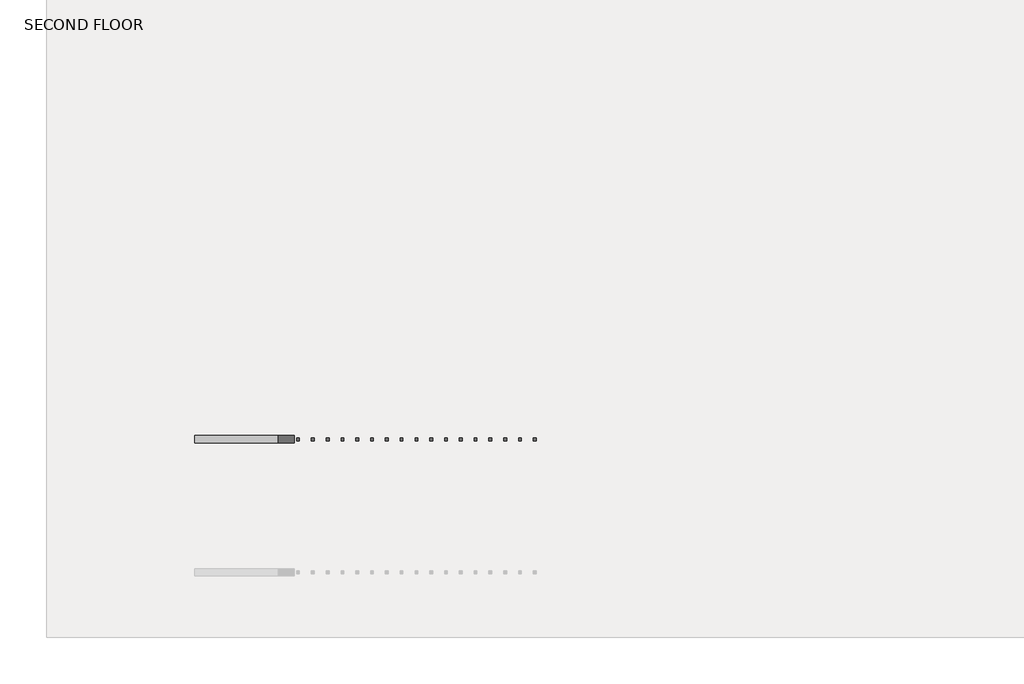
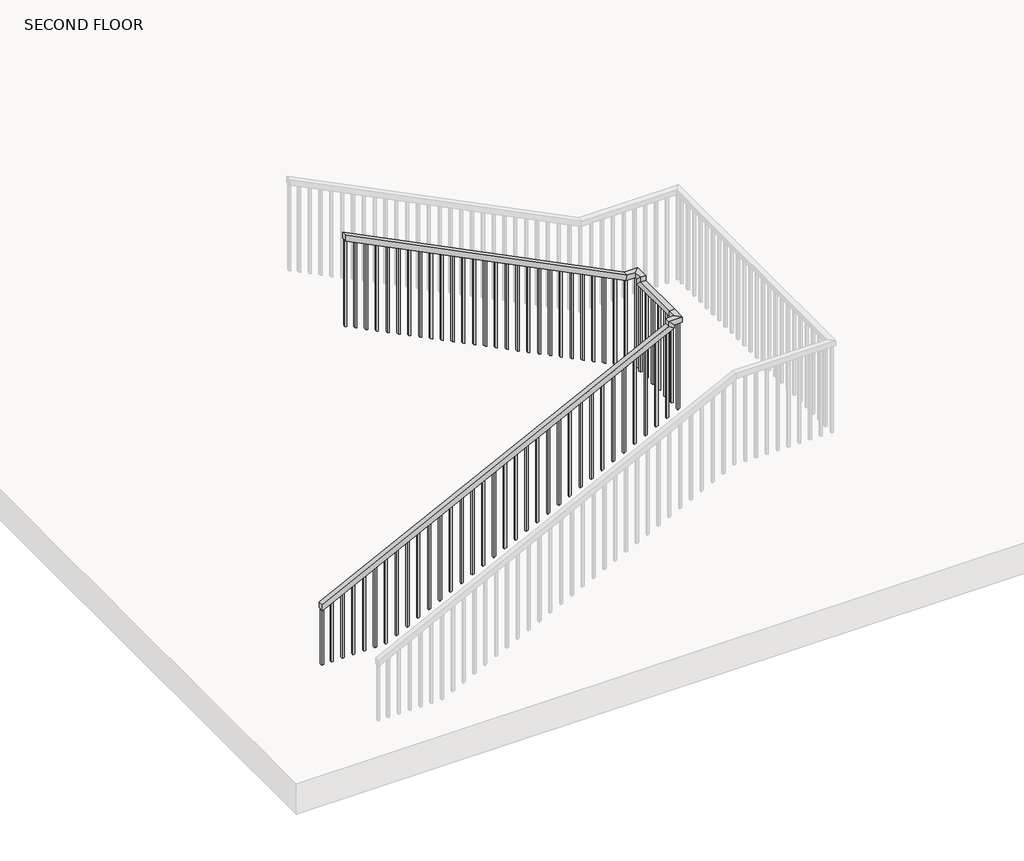
# One storey, part 2 of 2: 1 railing.
"""IFC4 building model written with IfcOpenShell, lengths in millimetres."""

from ifc_helpers import new_model, si_unit, frame, origin, place, context, project, spatial, polyline, outline, extrude, faceted_brep, element, save

model = new_model("IFC4")

# Units and contexts
model_context = context("Model", 3, world=origin())
ifc_project = project(units=[si_unit("LENGTHUNIT", "METRE", prefix="MILLI")], contexts=[model_context])

# Site, building, storey
site = spatial("IfcSite", under=ifc_project)
building = spatial("IfcBuilding", under=site)
storey = spatial("IfcBuildingStorey", under=building, Name="SECOND FLOOR", Elevation=6096.0)

# Railing
placement = place(None, origin())
element("IfcRailing", 1, ObjectType="Handrail - Rectangular", at=placement, inside=storey, context=model_context, shape_type="SolidModel", body=[
    faceted_brep([(-8362.2800418, -4455.7090076, 7010.4), (-8362.2800418, -4455.7090076, 6953.6038734), (-8362.2800418, -4506.5090076, 6953.6038734), (-8362.2800418, -4506.5090076, 7010.4), (-5111.0800418, -4455.7090076, 8636.0), (-5060.2800418, -4455.7090076, 8604.6038734), (-5060.2800418, -4506.5090076, 8604.6038734), (-5111.0800418, -4506.5090076, 8636.0), (-5111.0800418, -4455.7090076, 8686.8), (-5060.2800418, -4455.7090076, 8636.0), (-5060.2800418, -4506.5090076, 8636.0), (-5111.0800418, -4506.5090076, 8686.8), (-5034.8800418, -4455.7090076, 8686.8), (-5034.8800418, -4455.7090076, 8636.0), (-4984.0800418, -4506.5090076, 8636.0), (-4984.0800418, -4506.5090076, 8686.8), (-5034.8800418, -4379.5090076, 8686.8), (-5034.8800418, -4379.5090076, 8636.0), (-4984.0800418, -4379.5090076, 8636.0), (-4984.0800418, -4379.5090076, 8686.8), (-5034.8800418, -3907.7346494, 8686.8), (-5034.8800418, -3856.9346494, 8636.0), (-4984.0800418, -3856.9346494, 8636.0), (-4984.0800418, -3907.7346494, 8686.8), (-5034.8800418, -3907.7346494, 8737.6), (-5034.8800418, -3856.9346494, 8686.8), (-4984.0800418, -3856.9346494, 8686.8), (-4984.0800418, -3907.7346494, 8737.6), (-5034.8800418, -3831.5346494, 8737.6), (-5034.8800418, -3831.5346494, 8686.8), (-4984.0800418, -3780.7346494, 8686.8), (-4984.0800418, -3780.7346494, 8737.6), (-5111.0800418, -3831.5346494, 8737.6), (-5123.072295, -3831.5346494, 8686.8), (-5123.072295, -3780.7346494, 8686.8), (-5111.0800418, -3780.7346494, 8737.6), (-7752.6800418, -3831.5346494, 10058.4), (-7752.6800418, -3780.7346494, 10058.4), (-7752.6800418, -3780.7346494, 10001.6038734), (-7752.6800418, -3831.5346494, 10001.6038734)], [[[0, 1, 2, 3]], [[1, 0, 4, 5]], [[2, 1, 5, 6]], [[3, 2, 6, 7]], [[0, 3, 7, 4]], [[5, 4, 8, 9]], [[6, 5, 9, 10]], [[7, 6, 10, 11]], [[4, 7, 11, 8]], [[9, 8, 12, 13]], [[10, 9, 13, 14]], [[11, 10, 14, 15]], [[8, 11, 15, 12]], [[13, 12, 16, 17]], [[14, 13, 17, 18]], [[15, 14, 18, 19]], [[12, 15, 19, 16]], [[17, 16, 20, 21]], [[18, 17, 21, 22]], [[19, 18, 22, 23]], [[16, 19, 23, 20]], [[21, 20, 24, 25]], [[22, 21, 25, 26]], [[23, 22, 26, 27]], [[20, 23, 27, 24]], [[25, 24, 28, 29]], [[26, 25, 29, 30]], [[27, 26, 30, 31]], [[24, 27, 31, 28]], [[29, 28, 32, 33]], [[30, 29, 33, 34]], [[31, 30, 34, 35]], [[28, 31, 35, 32]], [[36, 37, 38, 39]], [[33, 32, 36, 39]], [[34, 33, 39, 38]], [[35, 34, 38, 37]], [[32, 35, 37, 36]]]),
    extrude(outline(polyline([(9946.0413734, -7641.5550418), (9955.5663734, -7660.6050418), (9097.9625, -7660.6050418), (9088.4375, -7641.5550418), (9946.0413734, -7641.5550418)])), frame((0.0, -3815.6596494, 0.0), z_axis=(0.0, 1.0, 0.0), x_axis=(0.0, 0.0, 1.0)), (0.0, 0.0, 1.0), 19.05),
    extrude(outline(polyline([(9895.2413734, -7539.9550418), (9904.7663734, -7559.0050418), (9047.1625, -7559.0050418), (9037.6375, -7539.9550418), (9895.2413734, -7539.9550418)])), frame((0.0, -3815.6596494, 0.0), z_axis=(0.0, 1.0, 0.0), x_axis=(0.0, 0.0, 1.0)), (0.0, 0.0, 1.0), 19.05),
    extrude(outline(polyline([(9844.4413734, -7438.3550418), (9853.9663734, -7457.4050418), (8996.3625, -7457.4050418), (8986.8375, -7438.3550418), (9844.4413734, -7438.3550418)])), frame((0.0, -3815.6596494, 0.0), z_axis=(0.0, 1.0, 0.0), x_axis=(0.0, 0.0, 1.0)), (0.0, 0.0, 1.0), 19.05),
    extrude(outline(polyline([(9793.6413734, -7336.7550418), (9803.1663734, -7355.8050418), (8945.5625, -7355.8050418), (8936.0375, -7336.7550418), (9793.6413734, -7336.7550418)])), frame((0.0, -3815.6596494, 0.0), z_axis=(0.0, 1.0, 0.0), x_axis=(0.0, 0.0, 1.0)), (0.0, 0.0, 1.0), 19.05),
    extrude(outline(polyline([(9742.8413734, -7235.1550418), (9752.3663734, -7254.2050418), (8894.7625, -7254.2050418), (8885.2375, -7235.1550418), (9742.8413734, -7235.1550418)])), frame((0.0, -3815.6596494, 0.0), z_axis=(0.0, 1.0, 0.0), x_axis=(0.0, 0.0, 1.0)), (0.0, 0.0, 1.0), 19.05),
    extrude(outline(polyline([(9692.0413734, -7133.5550418), (9701.5663734, -7152.6050418), (8843.9625, -7152.6050418), (8834.4375, -7133.5550418), (9692.0413734, -7133.5550418)])), frame((0.0, -3815.6596494, 0.0), z_axis=(0.0, 1.0, 0.0), x_axis=(0.0, 0.0, 1.0)), (0.0, 0.0, 1.0), 19.05),
    extrude(outline(polyline([(9641.2413734, -7031.9550418), (9650.7663734, -7051.0050418), (8793.1625, -7051.0050418), (8783.6375, -7031.9550418), (9641.2413734, -7031.9550418)])), frame((0.0, -3815.6596494, 0.0), z_axis=(0.0, 1.0, 0.0), x_axis=(0.0, 0.0, 1.0)), (0.0, 0.0, 1.0), 19.05),
    extrude(outline(polyline([(9590.4413734, -6930.3550418), (9599.9663734, -6949.4050418), (8742.3625, -6949.4050418), (8732.8375, -6930.3550418), (9590.4413734, -6930.3550418)])), frame((0.0, -3815.6596494, 0.0), z_axis=(0.0, 1.0, 0.0), x_axis=(0.0, 0.0, 1.0)), (0.0, 0.0, 1.0), 19.05),
    extrude(outline(polyline([(9539.6413734, -6828.7550418), (9549.1663734, -6847.8050418), (8691.5625, -6847.8050418), (8682.0375, -6828.7550418), (9539.6413734, -6828.7550418)])), frame((0.0, -3815.6596494, 0.0), z_axis=(0.0, 1.0, 0.0), x_axis=(0.0, 0.0, 1.0)), (0.0, 0.0, 1.0), 19.05),
    extrude(outline(polyline([(9488.8413734, -6727.1550418), (9498.3663734, -6746.2050418), (8640.7625, -6746.2050418), (8631.2375, -6727.1550418), (9488.8413734, -6727.1550418)])), frame((0.0, -3815.6596494, 0.0), z_axis=(0.0, 1.0, 0.0), x_axis=(0.0, 0.0, 1.0)), (0.0, 0.0, 1.0), 19.05),
    extrude(outline(polyline([(9438.0413734, -6625.5550418), (9447.5663734, -6644.6050418), (8589.9625, -6644.6050418), (8580.4375, -6625.5550418), (9438.0413734, -6625.5550418)])), frame((0.0, -3815.6596494, 0.0), z_axis=(0.0, 1.0, 0.0), x_axis=(0.0, 0.0, 1.0)), (0.0, 0.0, 1.0), 19.05),
    extrude(outline(polyline([(9387.2413734, -6523.9550418), (9396.7663734, -6543.0050418), (8539.1625, -6543.0050418), (8529.6375, -6523.9550418), (9387.2413734, -6523.9550418)])), frame((0.0, -3815.6596494, 0.0), z_axis=(0.0, 1.0, 0.0), x_axis=(0.0, 0.0, 1.0)), (0.0, 0.0, 1.0), 19.05),
    extrude(outline(polyline([(9336.4413734, -6422.3550418), (9345.9663734, -6441.4050418), (8488.3625, -6441.4050418), (8478.8375, -6422.3550418), (9336.4413734, -6422.3550418)])), frame((0.0, -3815.6596494, 0.0), z_axis=(0.0, 1.0, 0.0), x_axis=(0.0, 0.0, 1.0)), (0.0, 0.0, 1.0), 19.05),
    extrude(outline(polyline([(9285.6413734, -6320.7550418), (9295.1663734, -6339.8050418), (8437.5625, -6339.8050418), (8428.0375, -6320.7550418), (9285.6413734, -6320.7550418)])), frame((0.0, -3815.6596494, 0.0), z_axis=(0.0, 1.0, 0.0), x_axis=(0.0, 0.0, 1.0)), (0.0, 0.0, 1.0), 19.05),
    extrude(outline(polyline([(9234.8413734, -6219.1550418), (9244.3663734, -6238.2050418), (8386.7625, -6238.2050418), (8377.2375, -6219.1550418), (9234.8413734, -6219.1550418)])), frame((0.0, -3815.6596494, 0.0), z_axis=(0.0, 1.0, 0.0), x_axis=(0.0, 0.0, 1.0)), (0.0, 0.0, 1.0), 19.05),
    extrude(outline(polyline([(9184.0413734, -6117.5550418), (9193.5663734, -6136.6050418), (8335.9625, -6136.6050418), (8326.4375, -6117.5550418), (9184.0413734, -6117.5550418)])), frame((0.0, -3815.6596494, 0.0), z_axis=(0.0, 1.0, 0.0), x_axis=(0.0, 0.0, 1.0)), (0.0, 0.0, 1.0), 19.05),
    extrude(outline(polyline([(9133.2413734, -6015.9550418), (9142.7663734, -6035.0050418), (8285.1625, -6035.0050418), (8275.6375, -6015.9550418), (9133.2413734, -6015.9550418)])), frame((0.0, -3815.6596494, 0.0), z_axis=(0.0, 1.0, 0.0), x_axis=(0.0, 0.0, 1.0)), (0.0, 0.0, 1.0), 19.05),
    extrude(outline(polyline([(9082.4413734, -5914.3550418), (9091.9663734, -5933.4050418), (8234.3625, -5933.4050418), (8224.8375, -5914.3550418), (9082.4413734, -5914.3550418)])), frame((0.0, -3815.6596494, 0.0), z_axis=(0.0, 1.0, 0.0), x_axis=(0.0, 0.0, 1.0)), (0.0, 0.0, 1.0), 19.05),
    extrude(outline(polyline([(9031.6413734, -5812.7550418), (9041.1663734, -5831.8050418), (8183.5625, -5831.8050418), (8174.0375, -5812.7550418), (9031.6413734, -5812.7550418)])), frame((0.0, -3815.6596494, 0.0), z_axis=(0.0, 1.0, 0.0), x_axis=(0.0, 0.0, 1.0)), (0.0, 0.0, 1.0), 19.05),
    extrude(outline(polyline([(8980.8413734, -5711.1550418), (8990.3663734, -5730.2050418), (8132.7625, -5730.2050418), (8123.2375, -5711.1550418), (8980.8413734, -5711.1550418)])), frame((0.0, -3815.6596494, 0.0), z_axis=(0.0, 1.0, 0.0), x_axis=(0.0, 0.0, 1.0)), (0.0, 0.0, 1.0), 19.05),
    extrude(outline(polyline([(8930.0413734, -5609.5550418), (8939.5663734, -5628.6050418), (8081.9625, -5628.6050418), (8072.4375, -5609.5550418), (8930.0413734, -5609.5550418)])), frame((0.0, -3815.6596494, 0.0), z_axis=(0.0, 1.0, 0.0), x_axis=(0.0, 0.0, 1.0)), (0.0, 0.0, 1.0), 19.05),
    extrude(outline(polyline([(8879.2413734, -5507.9550418), (8888.7663734, -5527.0050418), (8031.1625, -5527.0050418), (8021.6375, -5507.9550418), (8879.2413734, -5507.9550418)])), frame((0.0, -3815.6596494, 0.0), z_axis=(0.0, 1.0, 0.0), x_axis=(0.0, 0.0, 1.0)), (0.0, 0.0, 1.0), 19.05),
    extrude(outline(polyline([(8828.4413734, -5406.3550418), (8837.9663734, -5425.4050418), (7980.3625, -5425.4050418), (7970.8375, -5406.3550418), (8828.4413734, -5406.3550418)])), frame((0.0, -3815.6596494, 0.0), z_axis=(0.0, 1.0, 0.0), x_axis=(0.0, 0.0, 1.0)), (0.0, 0.0, 1.0), 19.05),
    extrude(outline(polyline([(8777.6413734, -5304.7550418), (8787.1663734, -5323.8050418), (7929.5625, -5323.8050418), (7920.0375, -5304.7550418), (8777.6413734, -5304.7550418)])), frame((0.0, -3815.6596494, 0.0), z_axis=(0.0, 1.0, 0.0), x_axis=(0.0, 0.0, 1.0)), (0.0, 0.0, 1.0), 19.05),
    extrude(outline(polyline([(8726.8413734, -5203.1550418), (8736.3663734, -5222.2050418), (7878.7625, -5222.2050418), (7869.2375, -5203.1550418), (8726.8413734, -5203.1550418)])), frame((0.0, -3815.6596494, 0.0), z_axis=(0.0, 1.0, 0.0), x_axis=(0.0, 0.0, 1.0)), (0.0, 0.0, 1.0), 19.05),
    extrude(outline(polyline([(8686.8, -5101.5550418), (8686.8, -5120.6050418), (7827.9625, -5120.6050418), (7818.4375, -5101.5550418), (8686.8, -5101.5550418)])), frame((0.0, -3815.6596494, 0.0), z_axis=(0.0, 1.0, 0.0), x_axis=(0.0, 0.0, 1.0)), (0.0, 0.0, 1.0), 19.05),
    extrude(outline(polyline([(-4999.9550418, -3881.0340076), (-5019.0050418, -3881.0340076), (-5019.0050418, -3861.9840076), (-4999.9550418, -3861.9840076), (-4999.9550418, -3881.0340076)])), frame((0.0, 0.0, 7772.4), z_axis=(0.0, 0.0, 1.0), x_axis=(1.0, 0.0, 0.0)), (0.0, 0.0, 1.0), 863.6),
    extrude(outline(polyline([(-4999.9550418, -3982.6340076), (-5019.0050418, -3982.6340076), (-5019.0050418, -3963.5840076), (-4999.9550418, -3963.5840076), (-4999.9550418, -3982.6340076)])), frame((0.0, 0.0, 7772.4), z_axis=(0.0, 0.0, 1.0), x_axis=(1.0, 0.0, 0.0)), (0.0, 0.0, 1.0), 863.6),
    extrude(outline(polyline([(-4999.9550418, -4084.2340076), (-5019.0050418, -4084.2340076), (-5019.0050418, -4065.1840076), (-4999.9550418, -4065.1840076), (-4999.9550418, -4084.2340076)])), frame((0.0, 0.0, 7772.4), z_axis=(0.0, 0.0, 1.0), x_axis=(1.0, 0.0, 0.0)), (0.0, 0.0, 1.0), 863.6),
    extrude(outline(polyline([(-4999.9550418, -4185.8340076), (-5019.0050418, -4185.8340076), (-5019.0050418, -4166.7840076), (-4999.9550418, -4166.7840076), (-4999.9550418, -4185.8340076)])), frame((0.0, 0.0, 7772.4), z_axis=(0.0, 0.0, 1.0), x_axis=(1.0, 0.0, 0.0)), (0.0, 0.0, 1.0), 863.6),
    extrude(outline(polyline([(-4999.9550418, -4287.4340076), (-5019.0050418, -4287.4340076), (-5019.0050418, -4268.3840076), (-4999.9550418, -4268.3840076), (-4999.9550418, -4287.4340076)])), frame((0.0, 0.0, 7772.4), z_axis=(0.0, 0.0, 1.0), x_axis=(1.0, 0.0, 0.0)), (0.0, 0.0, 1.0), 863.6),
    extrude(outline(polyline([(-4999.9550418, -4389.0340076), (-5019.0050418, -4389.0340076), (-5019.0050418, -4369.9840076), (-4999.9550418, -4369.9840076), (-4999.9550418, -4389.0340076)])), frame((0.0, 0.0, 7772.4), z_axis=(0.0, 0.0, 1.0), x_axis=(1.0, 0.0, 0.0)), (0.0, 0.0, 1.0), 863.6),
    extrude(outline(polyline([(8583.9663734, -5101.5550418), (8574.4413734, -5120.6050418), (7716.8375, -5120.6050418), (7726.3625, -5101.5550418), (8583.9663734, -5101.5550418)])), frame((0.0, -4490.6340076, 0.0), z_axis=(0.0, 1.0, 0.0), x_axis=(0.0, 0.0, 1.0)), (0.0, 0.0, 1.0), 19.05),
    extrude(outline(polyline([(8533.1663734, -5203.1550418), (8523.6413734, -5222.2050418), (7666.0375, -5222.2050418), (7675.5625, -5203.1550418), (8533.1663734, -5203.1550418)])), frame((0.0, -4490.6340076, 0.0), z_axis=(0.0, 1.0, 0.0), x_axis=(0.0, 0.0, 1.0)), (0.0, 0.0, 1.0), 19.05),
    extrude(outline(polyline([(8482.3663734, -5304.7550418), (8472.8413734, -5323.8050418), (7615.2375, -5323.8050418), (7624.7625, -5304.7550418), (8482.3663734, -5304.7550418)])), frame((0.0, -4490.6340076, 0.0), z_axis=(0.0, 1.0, 0.0), x_axis=(0.0, 0.0, 1.0)), (0.0, 0.0, 1.0), 19.05),
    extrude(outline(polyline([(8431.5663734, -5406.3550418), (8422.0413734, -5425.4050418), (7564.4375, -5425.4050418), (7573.9625, -5406.3550418), (8431.5663734, -5406.3550418)])), frame((0.0, -4490.6340076, 0.0), z_axis=(0.0, 1.0, 0.0), x_axis=(0.0, 0.0, 1.0)), (0.0, 0.0, 1.0), 19.05),
    extrude(outline(polyline([(8380.7663734, -5507.9550418), (8371.2413734, -5527.0050418), (7513.6375, -5527.0050418), (7523.1625, -5507.9550418), (8380.7663734, -5507.9550418)])), frame((0.0, -4490.6340076, 0.0), z_axis=(0.0, 1.0, 0.0), x_axis=(0.0, 0.0, 1.0)), (0.0, 0.0, 1.0), 19.05),
    extrude(outline(polyline([(8329.9663734, -5609.5550418), (8320.4413734, -5628.6050418), (7462.8375, -5628.6050418), (7472.3625, -5609.5550418), (8329.9663734, -5609.5550418)])), frame((0.0, -4490.6340076, 0.0), z_axis=(0.0, 1.0, 0.0), x_axis=(0.0, 0.0, 1.0)), (0.0, 0.0, 1.0), 19.05),
    extrude(outline(polyline([(8279.1663734, -5711.1550418), (8269.6413734, -5730.2050418), (7412.0375, -5730.2050418), (7421.5625, -5711.1550418), (8279.1663734, -5711.1550418)])), frame((0.0, -4490.6340076, 0.0), z_axis=(0.0, 1.0, 0.0), x_axis=(0.0, 0.0, 1.0)), (0.0, 0.0, 1.0), 19.05),
    extrude(outline(polyline([(8228.3663734, -5812.7550418), (8218.8413734, -5831.8050418), (7361.2375, -5831.8050418), (7370.7625, -5812.7550418), (8228.3663734, -5812.7550418)])), frame((0.0, -4490.6340076, 0.0), z_axis=(0.0, 1.0, 0.0), x_axis=(0.0, 0.0, 1.0)), (0.0, 0.0, 1.0), 19.05),
    extrude(outline(polyline([(8177.5663734, -5914.3550418), (8168.0413734, -5933.4050418), (7310.4375, -5933.4050418), (7319.9625, -5914.3550418), (8177.5663734, -5914.3550418)])), frame((0.0, -4490.6340076, 0.0), z_axis=(0.0, 1.0, 0.0), x_axis=(0.0, 0.0, 1.0)), (0.0, 0.0, 1.0), 19.05),
    extrude(outline(polyline([(8126.7663734, -6015.9550418), (8117.2413734, -6035.0050418), (7259.6375, -6035.0050418), (7269.1625, -6015.9550418), (8126.7663734, -6015.9550418)])), frame((0.0, -4490.6340076, 0.0), z_axis=(0.0, 1.0, 0.0), x_axis=(0.0, 0.0, 1.0)), (0.0, 0.0, 1.0), 19.05),
    extrude(outline(polyline([(8075.9663734, -6117.5550418), (8066.4413734, -6136.6050418), (7208.8375, -6136.6050418), (7218.3625, -6117.5550418), (8075.9663734, -6117.5550418)])), frame((0.0, -4490.6340076, 0.0), z_axis=(0.0, 1.0, 0.0), x_axis=(0.0, 0.0, 1.0)), (0.0, 0.0, 1.0), 19.05),
    extrude(outline(polyline([(8025.1663734, -6219.1550418), (8015.6413734, -6238.2050418), (7158.0375, -6238.2050418), (7167.5625, -6219.1550418), (8025.1663734, -6219.1550418)])), frame((0.0, -4490.6340076, 0.0), z_axis=(0.0, 1.0, 0.0), x_axis=(0.0, 0.0, 1.0)), (0.0, 0.0, 1.0), 19.05),
    extrude(outline(polyline([(7974.3663734, -6320.7550418), (7964.8413734, -6339.8050418), (7107.2375, -6339.8050418), (7116.7625, -6320.7550418), (7974.3663734, -6320.7550418)])), frame((0.0, -4490.6340076, 0.0), z_axis=(0.0, 1.0, 0.0), x_axis=(0.0, 0.0, 1.0)), (0.0, 0.0, 1.0), 19.05),
    extrude(outline(polyline([(7923.5663734, -6422.3550418), (7914.0413734, -6441.4050418), (7056.4375, -6441.4050418), (7065.9625, -6422.3550418), (7923.5663734, -6422.3550418)])), frame((0.0, -4490.6340076, 0.0), z_axis=(0.0, 1.0, 0.0), x_axis=(0.0, 0.0, 1.0)), (0.0, 0.0, 1.0), 19.05),
    extrude(outline(polyline([(7872.7663734, -6523.9550418), (7863.2413734, -6543.0050418), (7005.6375, -6543.0050418), (7015.1625, -6523.9550418), (7872.7663734, -6523.9550418)])), frame((0.0, -4490.6340076, 0.0), z_axis=(0.0, 1.0, 0.0), x_axis=(0.0, 0.0, 1.0)), (0.0, 0.0, 1.0), 19.05),
    extrude(outline(polyline([(7821.9663734, -6625.5550418), (7812.4413734, -6644.6050418), (6954.8375, -6644.6050418), (6964.3625, -6625.5550418), (7821.9663734, -6625.5550418)])), frame((0.0, -4490.6340076, 0.0), z_axis=(0.0, 1.0, 0.0), x_axis=(0.0, 0.0, 1.0)), (0.0, 0.0, 1.0), 19.05),
    extrude(outline(polyline([(7771.1663734, -6727.1550418), (7761.6413734, -6746.2050418), (6904.0375, -6746.2050418), (6913.5625, -6727.1550418), (7771.1663734, -6727.1550418)])), frame((0.0, -4490.6340076, 0.0), z_axis=(0.0, 1.0, 0.0), x_axis=(0.0, 0.0, 1.0)), (0.0, 0.0, 1.0), 19.05),
    extrude(outline(polyline([(7720.3663734, -6828.7550418), (7710.8413734, -6847.8050418), (6853.2375, -6847.8050418), (6862.7625, -6828.7550418), (7720.3663734, -6828.7550418)])), frame((0.0, -4490.6340076, 0.0), z_axis=(0.0, 1.0, 0.0), x_axis=(0.0, 0.0, 1.0)), (0.0, 0.0, 1.0), 19.05),
    extrude(outline(polyline([(7669.5663734, -6930.3550418), (7660.0413734, -6949.4050418), (6802.4375, -6949.4050418), (6811.9625, -6930.3550418), (7669.5663734, -6930.3550418)])), frame((0.0, -4490.6340076, 0.0), z_axis=(0.0, 1.0, 0.0), x_axis=(0.0, 0.0, 1.0)), (0.0, 0.0, 1.0), 19.05),
    extrude(outline(polyline([(7618.7663734, -7031.9550418), (7609.2413734, -7051.0050418), (6751.6375, -7051.0050418), (6761.1625, -7031.9550418), (7618.7663734, -7031.9550418)])), frame((0.0, -4490.6340076, 0.0), z_axis=(0.0, 1.0, 0.0), x_axis=(0.0, 0.0, 1.0)), (0.0, 0.0, 1.0), 19.05),
    extrude(outline(polyline([(7567.9663734, -7133.5550418), (7558.4413734, -7152.6050418), (6700.8375, -7152.6050418), (6710.3625, -7133.5550418), (7567.9663734, -7133.5550418)])), frame((0.0, -4490.6340076, 0.0), z_axis=(0.0, 1.0, 0.0), x_axis=(0.0, 0.0, 1.0)), (0.0, 0.0, 1.0), 19.05),
    extrude(outline(polyline([(7517.1663734, -7235.1550418), (7507.6413734, -7254.2050418), (6650.0375, -7254.2050418), (6659.5625, -7235.1550418), (7517.1663734, -7235.1550418)])), frame((0.0, -4490.6340076, 0.0), z_axis=(0.0, 1.0, 0.0), x_axis=(0.0, 0.0, 1.0)), (0.0, 0.0, 1.0), 19.05),
    extrude(outline(polyline([(7466.3663734, -7336.7550418), (7456.8413734, -7355.8050418), (6599.2375, -7355.8050418), (6608.7625, -7336.7550418), (7466.3663734, -7336.7550418)])), frame((0.0, -4490.6340076, 0.0), z_axis=(0.0, 1.0, 0.0), x_axis=(0.0, 0.0, 1.0)), (0.0, 0.0, 1.0), 19.05),
    extrude(outline(polyline([(7415.5663734, -7438.3550418), (7406.0413734, -7457.4050418), (6548.4375, -7457.4050418), (6557.9625, -7438.3550418), (7415.5663734, -7438.3550418)])), frame((0.0, -4490.6340076, 0.0), z_axis=(0.0, 1.0, 0.0), x_axis=(0.0, 0.0, 1.0)), (0.0, 0.0, 1.0), 19.05),
    extrude(outline(polyline([(7364.7663734, -7539.9550418), (7355.2413734, -7559.0050418), (6497.6375, -7559.0050418), (6507.1625, -7539.9550418), (7364.7663734, -7539.9550418)])), frame((0.0, -4490.6340076, 0.0), z_axis=(0.0, 1.0, 0.0), x_axis=(0.0, 0.0, 1.0)), (0.0, 0.0, 1.0), 19.05),
    extrude(outline(polyline([(7313.9663734, -7641.5550418), (7304.4413734, -7660.6050418), (6446.8375, -7660.6050418), (6456.3625, -7641.5550418), (7313.9663734, -7641.5550418)])), frame((0.0, -4490.6340076, 0.0), z_axis=(0.0, 1.0, 0.0), x_axis=(0.0, 0.0, 1.0)), (0.0, 0.0, 1.0), 19.05),
    extrude(outline(polyline([(7263.1663734, -7743.1550418), (7253.6413734, -7762.2050418), (6396.0375, -7762.2050418), (6405.5625, -7743.1550418), (7263.1663734, -7743.1550418)])), frame((0.0, -4490.6340076, 0.0), z_axis=(0.0, 1.0, 0.0), x_axis=(0.0, 0.0, 1.0)), (0.0, 0.0, 1.0), 19.05),
    extrude(outline(polyline([(7212.3663734, -7844.7550418), (7202.8413734, -7863.8050418), (6345.2375, -7863.8050418), (6354.7625, -7844.7550418), (7212.3663734, -7844.7550418)])), frame((0.0, -4490.6340076, 0.0), z_axis=(0.0, 1.0, 0.0), x_axis=(0.0, 0.0, 1.0)), (0.0, 0.0, 1.0), 19.05),
    extrude(outline(polyline([(7161.5663734, -7946.3550418), (7152.0413734, -7965.4050418), (6294.4375, -7965.4050418), (6303.9625, -7946.3550418), (7161.5663734, -7946.3550418)])), frame((0.0, -4490.6340076, 0.0), z_axis=(0.0, 1.0, 0.0), x_axis=(0.0, 0.0, 1.0)), (0.0, 0.0, 1.0), 19.05),
    extrude(outline(polyline([(7110.7663734, -8047.9550418), (7101.2413734, -8067.0050418), (6243.6375, -8067.0050418), (6253.1625, -8047.9550418), (7110.7663734, -8047.9550418)])), frame((0.0, -4490.6340076, 0.0), z_axis=(0.0, 1.0, 0.0), x_axis=(0.0, 0.0, 1.0)), (0.0, 0.0, 1.0), 19.05),
    extrude(outline(polyline([(7059.9663734, -8149.5550418), (7050.4413734, -8168.6050418), (6192.8375, -8168.6050418), (6202.3625, -8149.5550418), (7059.9663734, -8149.5550418)])), frame((0.0, -4490.6340076, 0.0), z_axis=(0.0, 1.0, 0.0), x_axis=(0.0, 0.0, 1.0)), (0.0, 0.0, 1.0), 19.05),
    extrude(outline(polyline([(7009.1663734, -8251.1550418), (6999.6413734, -8270.2050418), (6142.0375, -8270.2050418), (6151.5625, -8251.1550418), (7009.1663734, -8251.1550418)])), frame((0.0, -4490.6340076, 0.0), z_axis=(0.0, 1.0, 0.0), x_axis=(0.0, 0.0, 1.0)), (0.0, 0.0, 1.0), 19.05),
    extrude(outline(polyline([(-4999.9550418, -3815.6596494), (-5019.0050418, -3815.6596494), (-5019.0050418, -3796.6096494), (-4999.9550418, -3796.6096494), (-4999.9550418, -3815.6596494)])), frame((0.0, 0.0, 7772.4), z_axis=(0.0, 0.0, 1.0), x_axis=(1.0, 0.0, 0.0)), (0.0, 0.0, 1.0), 914.4),
    extrude(outline(polyline([(8636.0, -4999.9550418), (8636.0, -5019.0050418), (7767.6375, -5019.0050418), (7777.1625, -4999.9550418), (8636.0, -4999.9550418)])), frame((0.0, -4490.6340076, 0.0), z_axis=(0.0, 1.0, 0.0), x_axis=(0.0, 0.0, 1.0)), (0.0, 0.0, 1.0), 19.05),
    extrude(outline(polyline([(9992.0788734, -7733.6300418), (10001.6038734, -7752.6800418), (9144.0, -7752.6800418), (9134.475, -7733.6300418), (9992.0788734, -7733.6300418)])), frame((0.0, -3815.6596494, 0.0), z_axis=(0.0, 1.0, 0.0), x_axis=(0.0, 0.0, 1.0)), (0.0, 0.0, 1.0), 19.05),
    extrude(outline(polyline([(6963.1288734, -8343.2300418), (6953.6038734, -8362.2800418), (6096.0, -8362.2800418), (6105.525, -8343.2300418), (6963.1288734, -8343.2300418)])), frame((0.0, -4490.6340076, 0.0), z_axis=(0.0, 1.0, 0.0), x_axis=(0.0, 0.0, 1.0)), (0.0, 0.0, 1.0), 19.05),
])

save(model, "model.ifc")

# Revit data of these elements
# Type "Handrail - Rectangular"
#   Assembly Code = "C2010400"
#   built-in parameter 1008612 = 0.0416667 (stored number, unit not read)
#   built-in parameter 1008611 = 0.0416667 (stored number, unit not read)
#   built-in parameter 1008609 = 0.333333 (stored number, unit not read)
#   built-in parameter 1008604 = 0.166667 (stored number, unit not read)
#   built-in parameter 1008603 = 0.166667 (stored number, unit not read)
#   Railing Height = 3' - 0"
#   built-in parameter 1008630 = 2
#   built-in parameter 1008610 = 2
#   built-in parameter 1008618 = Baluster - Square : 3/4"
# Element 1 (IfcRailing, "Handrail - Rectangular")
#   Phase Created = New Construction
